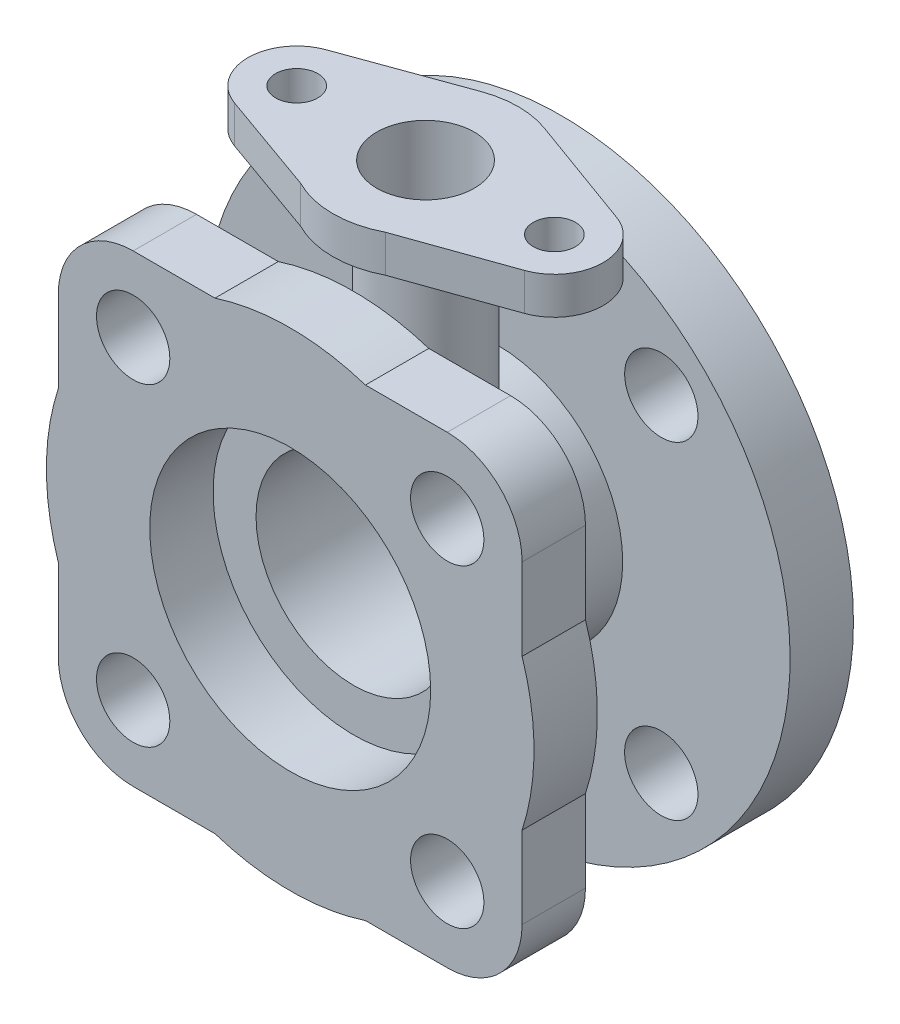
from build123d import *

# Parameters (mm, degrees)
ROUND_FLANGE_SKETCH_R                 = 76.2
ROUND_FLANGE_152_4_DEPTH              = 16.5
HUB_SKETCH_R                          = 32.6
HUB_65_2_DEPTH                        = 18.75
TAPERED_NECK_SKETCH_R                 = 32.6
TAPERED_NECK_12DEG_DRAFT_DEPTH        = 18.75
TAPERED_NECK_12DEG_DRAFT_DRAFT        = -12
SQUARE_FLANGE_SKETCH_R                = 36.585435531
SQUARE_FLANGE_127_DEPTH               = 16.5
SQUARE_FLANGE_HOLES_SKETCH_R          = 9.55
SQUARE_FLANGE_HOLES_DEPTH             = 20.5
ROUND_FLANGE_BOLT_HOLES_SKETCH_R      = 9.55
ROUND_FLANGE_BOLT_HOLES_4X_19_1_DEPTH = 20.5
SQUARE_FLANGE_BORE_SKETCH_R           = 25.4
SQUARE_FLANGE_BORE_DEPTH              = 121
SIDE_PORT_BOSS_SKETCH_R               = 13.5
SIDE_PORT_BOSS_DEPTH                  = 74
PORT_PAD_DEPTH                        = 9.7
ROUND_FLANGE_BORE_SKETCH_R            = 25.4
ROUND_FLANGE_BORE_DEPTH               = 352.7
PAD_BOLT_HOLES_SKETCH_R               = 5.5
PAD_BOLT_HOLES_2X_DEPTH               = 32.7
SIDE_PORT_BORE_SKETCH_R               = 12.7
SIDE_PORT_BORE_DEPTH                  = 74.7


with BuildPart() as part:
    # Round Flange Sketch → Round Flange Ø152.4 (new body)
    with BuildSketch(Plane.XY):
        Circle(ROUND_FLANGE_SKETCH_R)
    extrude(amount=ROUND_FLANGE_152_4_DEPTH)

    # Hub Sketch → Hub Ø65.2 (add)
    with BuildSketch(Plane.XY.offset(16.5)):
        Circle(HUB_SKETCH_R)
    extrude(amount=HUB_65_2_DEPTH)


with BuildPart() as tapered_neck_12deg_draft_tool:
    # Tapered Neck Sketch → Tapered Neck 12deg Draft (with draft: the straight prism first)
    with BuildSketch(Plane.XY.offset(35.25)):
        Circle(TAPERED_NECK_SKETCH_R)
    extrude(amount=TAPERED_NECK_12DEG_DRAFT_DEPTH)
    # Tapered Neck 12deg Draft: the draft: its side faces are tilted about the plane it starts from
    tapered_neck_12deg_draft_sides = [tapered_neck_12deg_draft_tool.faces().sort_by_distance(p)[0] for p in [
        (-32.6, 0, 44.625),
    ]]
    draft(tapered_neck_12deg_draft_sides, Plane.XY.offset(35.25), TAPERED_NECK_12DEG_DRAFT_DRAFT)


with BuildPart() as part_1:
    add(part.part)

    # Tapered Neck 12deg Draft: add tapered_neck_12deg_draft_tool
    add(tapered_neck_12deg_draft_tool.part)

    # Round Flange Bolt Holes Sketch → Round Flange Bolt Holes 4xØ19.1 (cut)
    with BuildSketch(Plane(origin=(0, 0, 0), x_dir=(-1, 0, 0), z_dir=(0, 0, -1))):
        with Locations((42.65, -42.65)):
            Circle(ROUND_FLANGE_BOLT_HOLES_SKETCH_R)
        with Locations(Location((42.65, 42.65, 0), (0, 0, 180))):
            Circle(ROUND_FLANGE_BOLT_HOLES_SKETCH_R)
        with Locations(Location((-42.65, -42.65, 0), (0, 0, 180))):
            Circle(ROUND_FLANGE_BOLT_HOLES_SKETCH_R)
        with Locations((-42.65, 42.65)):
            Circle(ROUND_FLANGE_BOLT_HOLES_SKETCH_R)
    extrude(amount=-ROUND_FLANGE_BOLT_HOLES_4X_19_1_DEPTH, mode=Mode.SUBTRACT)

    # Square Flange Bore Sketch → Square Flange Bore (cut)
    with BuildSketch(Plane.XY.offset(70.5)):
        Circle(SQUARE_FLANGE_BORE_SKETCH_R)
    extrude(amount=-SQUARE_FLANGE_BORE_DEPTH, mode=Mode.SUBTRACT)

    # Side Port Boss Sketch → Side Port Boss (add)
    with BuildSketch(Plane(origin=(0, 0, 0), x_dir=(1, 0, 0), z_dir=(0, 1, 0))):
        with Locations(Location((0, -35.25, 0), (0, 0, 90))):
            Circle(SIDE_PORT_BOSS_SKETCH_R)
    extrude(amount=SIDE_PORT_BOSS_DEPTH)

    # Port Pad Sketch → Port Pad (add)
    with BuildSketch(Plane(origin=(0, 74, 0), x_dir=(1, 0, 0), z_dir=(0, 1, 0))):
        with BuildLine():
            Line((-37.884277198, -23.312494349), (-8.24195231, -12.549940041))
            ThreePointArc((-8.24195231, -12.549940041), (0, -11.1), (8.24195231, -12.549940041))
            Line((8.24195231, -12.549940041), (37.884277198, -23.312494349))
            ThreePointArc((37.884277198, -23.312494349), (46.249722111, -35.334013693), (37.725962102, -47.243804256))
            Line((37.725962102, -47.243804256), (11.009644458, -56.744423205))
            ThreePointArc((11.009644458, -56.744423205), (0, -59.4), (-11.009644458, -56.744423205))
            Line((-11.009644458, -56.744423205), (-37.884277198, -47.187505651))
            ThreePointArc((-37.884277198, -47.187505651), (-46.25, -35.25), (-37.884277198, -23.312494349))
        make_face()
    extrude(amount=PORT_PAD_DEPTH)

    # Round Flange Bore Sketch → Round Flange Bore (cut)
    with BuildSketch(Plane.XY.offset(54)):
        Circle(ROUND_FLANGE_BORE_SKETCH_R)
    extrude(amount=-ROUND_FLANGE_BORE_DEPTH, mode=Mode.SUBTRACT)

    # Pad Bolt Holes Sketch → Pad Bolt Holes 2x (cut)
    with BuildSketch(Plane(origin=(0, 83.7, 0), x_dir=(1, 0, 0), z_dir=(0, 1, 0))):
        with Locations(Location((33.55, -35.25, 0), (0, 0, 270))):
            Circle(PAD_BOLT_HOLES_SKETCH_R)
        with Locations(Location((-33.55, -35.25, 0), (0, 0, 270))):
            Circle(PAD_BOLT_HOLES_SKETCH_R)
    extrude(amount=-PAD_BOLT_HOLES_2X_DEPTH, mode=Mode.SUBTRACT)

    # Side Port Bore Sketch → Side Port Bore (cut)
    with BuildSketch(Plane(origin=(0, 83.7, 0), x_dir=(1, 0, 0), z_dir=(0, 1, 0))):
        with Locations(Location((0, -35.25, 0), (0, 0, 270))):
            Circle(SIDE_PORT_BORE_SKETCH_R)
    extrude(amount=-SIDE_PORT_BORE_DEPTH, mode=Mode.SUBTRACT)


with BuildPart() as body_2:
    # Square Flange Sketch → Square Flange 127 (new body)
    with BuildSketch(Plane.XY.offset(54)):
        with BuildLine():
            Line((-40.9, -60.4), (-19.598214204, -60.4))
            ThreePointArc((-19.598214204, -60.4), (0, -63.5), (19.598214204, -60.4))
            Line((19.598214204, -60.4), (40.9, -60.4))
            ThreePointArc((40.9, -60.4), (54.688582233, -54.688582233), (60.4, -40.9))
            Line((60.4, -40.9), (60.4, -19.598214204))
            ThreePointArc((60.4, -19.598214204), (63.5, 0), (60.4, 19.598214204))
            Line((60.4, 19.598214204), (60.4, 40.9))
            ThreePointArc((60.4, 40.9), (54.688582233, 54.688582233), (40.9, 60.4))
            Line((40.9, 60.4), (19.598214204, 60.4))
            ThreePointArc((19.598214204, 60.4), (0, 63.5), (-19.598214204, 60.4))
            Line((-19.598214204, 60.4), (-40.9, 60.4))
            ThreePointArc((-40.9, 60.4), (-54.688582233, 54.688582233), (-60.4, 40.9))
            Line((-60.4, 40.9), (-60.4, 19.598214204))
            ThreePointArc((-60.4, 19.598214204), (-63.5, 0), (-60.4, -19.598214204))
            Line((-60.4, -19.598214204), (-60.4, -40.9))
            ThreePointArc((-60.4, -40.9), (-54.688582233, -54.688582233), (-40.9, -60.4))
        make_face()
        Circle(SQUARE_FLANGE_SKETCH_R, mode=Mode.SUBTRACT)
    extrude(amount=SQUARE_FLANGE_127_DEPTH)

    # Square Flange Holes Sketch → Square Flange Holes (cut)
    with BuildSketch(Plane.XY.offset(70.5)):
        with Locations((-40.9, 40.9)):
            Circle(SQUARE_FLANGE_HOLES_SKETCH_R)
        with Locations((40.9, 40.9)):
            Circle(SQUARE_FLANGE_HOLES_SKETCH_R)
        with Locations((40.9, -40.9)):
            Circle(SQUARE_FLANGE_HOLES_SKETCH_R)
        with Locations((-40.9, -40.9)):
            Circle(SQUARE_FLANGE_HOLES_SKETCH_R)
    extrude(amount=-SQUARE_FLANGE_HOLES_DEPTH, mode=Mode.SUBTRACT)


solid = Compound([part_1.part, body_2.part])
